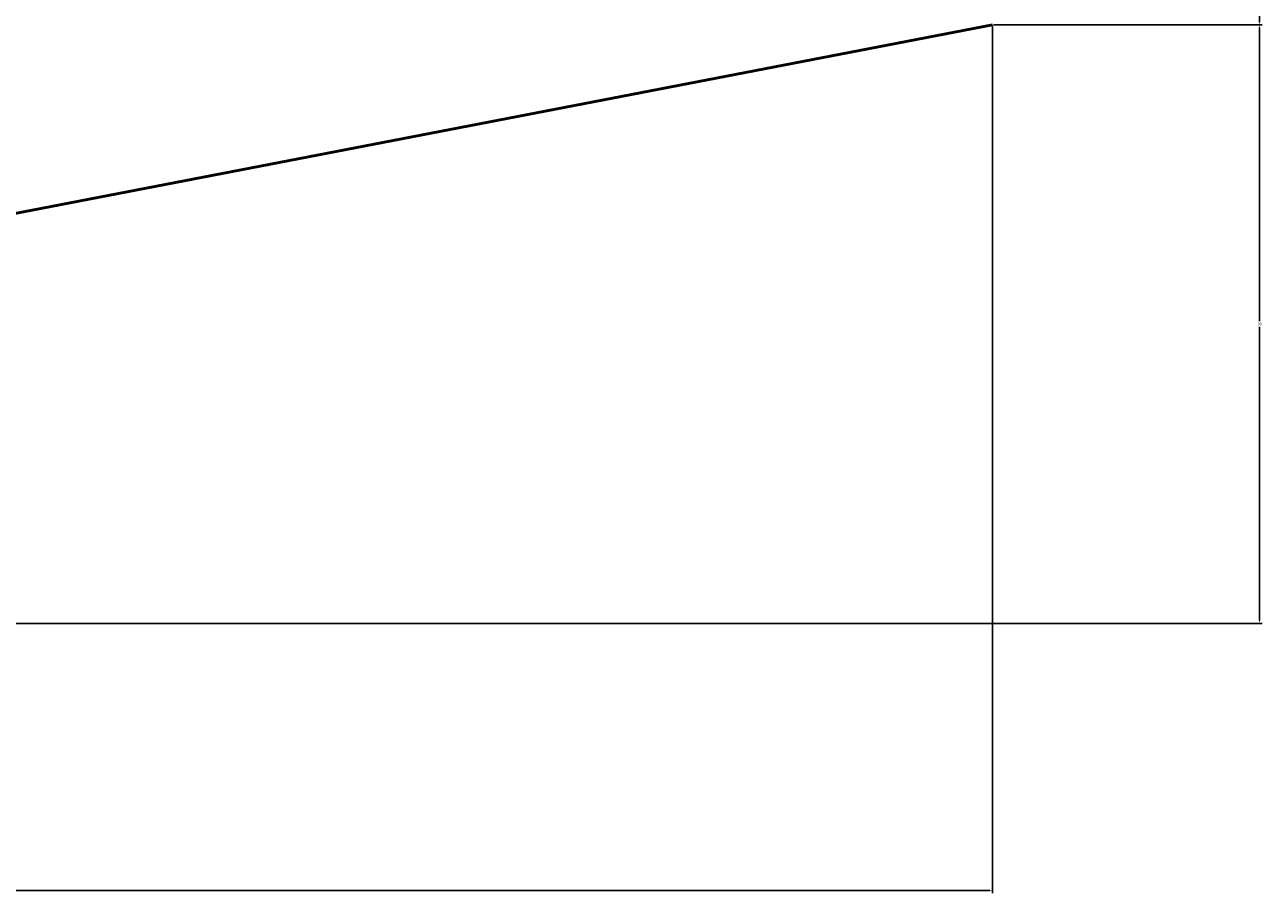
# Model space of a CAD drawing. Units: inches. Extents: x 457 to 775, y 319 to 541.
# Tile 9 of 12: x 694 to 775, y 319 to 376. Entities that reach past the tile are written whole.
import ezdxf

# ---------------------------------------------------------------- set-up
doc = ezdxf.new("R2010")
doc.units = ezdxf.units.IN
doc.header["$MEASUREMENT"] = 0
doc.layers.add('M-DIMS', color=2, linetype='Continuous', lineweight=18)
doc.layers.add('M-OUTL', color=7, linetype='Continuous', lineweight=50)
doc.styles.get("Standard").update_dxf_attribs({"font": 'arial.ttf'})
doc.dimstyles.get("Standard").update_dxf_attribs({"dimtxt": 0.18, "dimasz": 0.18, "dimexe": 0.18, "dimexo": 0.0625, "dimgap": 0.09, "dimtad": 0, "dimtih": 1, "dimtoh": 1, "dimdec": 4, "dimzin": 0, "dimdsep": 46, "dimtxsty": 'Standard', "dimcen": 0.09, "dimadec": 0, "dimazin": 0, "dimtfac": 1, "dimtdec": 4, "dimtofl": 0, "dimtmove": 0, "dimatfit": 3, "dimfxl": 1, "dimtolj": 1, "dimtzin": 0, "dimarcsym": 0})

# ---------------------------------------------------------------- blocks, each defined once
blk = doc.blocks.new('*D2')
at = {"layer": 'Defpoints', "color": 0, "transparency": 16777216}
for p in [(756.931, 375.696), (474.306, 336.696), (756.931, 319.296)]:
    blk.add_point(p, dxfattribs=at)
at = {"layer": 'M-DIMS', "color": 0, "lineweight": -2, "transparency": 16777216}
for p, q in [((756.931, 375.634), (756.931, 319.116)), ((474.306, 336.634), (474.306, 319.116)), ((474.486, 319.296), (615.223, 319.296)), ((756.751, 319.296), (616.014, 319.296))]:
    blk.add_line(p, q, dxfattribs=at)
at = {"layer": 'M-DIMS', "color": 0, "transparency": 16777216}
for points in [[(474.486, 319.326), (474.486, 319.266), (474.306, 319.296)], [(756.751, 319.326), (756.751, 319.266), (756.931, 319.296)]]:
    blk.add_solid(points, dxfattribs=at)
at = {"layer": 'M-DIMS', "color": 0, "transparency": 16777216, "insert": (615.619, 319.296), "char_height": 0.18, "attachment_point": 5}
blk.add_mtext('\\A1;282.6', dxfattribs=at)
blk = doc.blocks.new('*D9')
at = {"layer": 'Defpoints', "color": 0, "transparency": 16777216}
for p in [(756.931, 375.696), (774.331, 375.696), (554.931, 336.696)]:
    blk.add_point(p, dxfattribs=at)
at = {"layer": 'M-DIMS', "color": 0, "lineweight": -2, "transparency": 16777216}
for p, q in [((756.994, 375.696), (774.511, 375.696)), ((774.331, 375.516), (774.331, 356.378)), ((774.331, 336.876), (774.331, 356.014)), ((554.994, 336.696), (774.511, 336.696))]:
    blk.add_line(p, q, dxfattribs=at)
at = {"layer": 'M-DIMS', "color": 0, "transparency": 16777216}
for points in [[(774.301, 375.516), (774.361, 375.516), (774.331, 375.696)], [(774.301, 336.876), (774.361, 336.876), (774.331, 336.696)]]:
    blk.add_solid(points, dxfattribs=at)
at = {"layer": 'M-DIMS', "color": 0, "transparency": 16777216, "insert": (774.331, 356.196), "char_height": 0.18, "attachment_point": 5}
blk.add_mtext('\\A1;39', dxfattribs=at)
blk = doc.blocks.new('*D15')
at = {"layer": 'Defpoints', "color": 0, "transparency": 16777216}
for p in [(731.931, 388.196), (756.931, 375.696), (774.331, 375.696)]:
    blk.add_point(p, dxfattribs=at)
at = {"layer": 'M-DIMS', "color": 0, "lineweight": -2, "transparency": 16777216}
for p, q in [((731.994, 388.196), (774.511, 388.196)), ((774.331, 388.016), (774.331, 382.128)), ((774.331, 375.876), (774.331, 381.764)), ((756.994, 375.696), (774.511, 375.696))]:
    blk.add_line(p, q, dxfattribs=at)
at = {"layer": 'M-DIMS', "color": 0, "transparency": 16777216}
for points in [[(774.301, 388.016), (774.361, 388.016), (774.331, 388.196)], [(774.301, 375.876), (774.361, 375.876), (774.331, 375.696)]]:
    blk.add_solid(points, dxfattribs=at)
at = {"layer": 'M-DIMS', "color": 0, "transparency": 16777216, "insert": (774.331, 381.946), "char_height": 0.18, "attachment_point": 5}
blk.add_mtext('\\A1;12.5', dxfattribs=at)

msp = doc.modelspace()

# ---------------------------------------------------------------- linework, layer by layer
at = {"layer": 'M-OUTL'}
msp.add_line((554.931, 336.696), (756.931, 375.696), dxfattribs=at)

# ---------------------------------------------------------------- dimensions: what is measured, and where the dimension line sits
at = {"layer": 'M-DIMS'}
for p1, override, picture, middle in [((731.931, 388.196), {"dimdec": 1, "dimlfac": 1, "dimrnd": 0, "dimzin": 0, "dimdsep": 46, "dimlunit": 2}, '*D15', (774.331, 381.946)), ((554.931, 336.696), {"dimdec": 0, "dimlfac": 1, "dimrnd": 0, "dimzin": 0, "dimdsep": 46, "dimlunit": 2}, '*D9', (774.331, 356.196))]:
    dim = msp.add_linear_dim(base=(774.331, 375.696), p1=p1, p2=(756.931, 375.696), angle=90, dimstyle='Standard', override=override, dxfattribs=at)
    dim.commit()
    dim.dimension.update_dxf_attribs({"geometry": picture, "text_midpoint": middle})
dim = msp.add_linear_dim(base=(756.931, 319.296), p1=(474.306, 336.696), p2=(756.931, 375.696), dimstyle='Standard', override={"dimdec": 1, "dimlfac": 1, "dimrnd": 0, "dimzin": 0, "dimdsep": 46, "dimlunit": 2}, dxfattribs=at)
dim.commit()
dim.dimension.update_dxf_attribs({"geometry": '*D2', "text_midpoint": (615.619, 319.296)})

doc.saveas('drawing.dxf')
